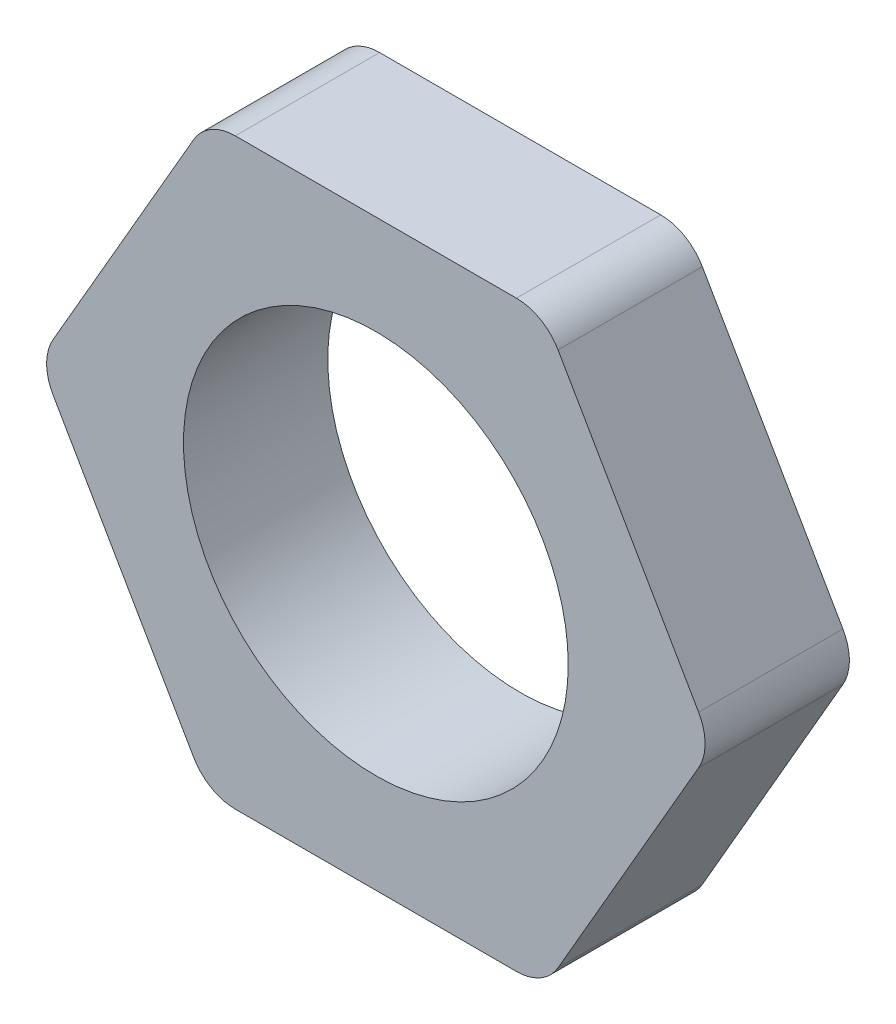
ISO-10303-21;
HEADER;
FILE_DESCRIPTION(('STEP AP214'),'2;1');
FILE_NAME('part.step','',(''),(''),'','','');
FILE_SCHEMA(('AUTOMOTIVE_DESIGN { 1 0 10303 214 1 1 1 1 }'));
ENDSEC;
DATA;
#1=APPLICATION_CONTEXT('core data for automotive mechanical design processes');
#2=APPLICATION_PROTOCOL_DEFINITION('international standard','automotive_design',2000,#1);
#3=PRODUCT_CONTEXT('',#1,'mechanical');
#4=PRODUCT('Part','Part','',(#3));
#5=PRODUCT_RELATED_PRODUCT_CATEGORY('part','',(#4));
#6=PRODUCT_DEFINITION_FORMATION('','',#4);
#7=PRODUCT_DEFINITION_CONTEXT('part definition',#1,'design');
#8=PRODUCT_DEFINITION('design','',#6,#7);
#9=PRODUCT_DEFINITION_SHAPE('','',#8);
#10=(LENGTH_UNIT() NAMED_UNIT(*) SI_UNIT(.MILLI.,.METRE.));
#11=(NAMED_UNIT(*) PLANE_ANGLE_UNIT() SI_UNIT($,.RADIAN.));
#12=(NAMED_UNIT(*) SI_UNIT($,.STERADIAN.) SOLID_ANGLE_UNIT());
#13=UNCERTAINTY_MEASURE_WITH_UNIT(LENGTH_MEASURE(1.E-05),#10,'distance_accuracy_value','');
#14=(GEOMETRIC_REPRESENTATION_CONTEXT(3) GLOBAL_UNCERTAINTY_ASSIGNED_CONTEXT((#13)) GLOBAL_UNIT_ASSIGNED_CONTEXT((#10,
#11,#12)) REPRESENTATION_CONTEXT('',''));
#15=CARTESIAN_POINT('',(0.,0.,0.));
#16=DIRECTION('',(0.,0.,1.));
#17=DIRECTION('',(1.,0.,0.));
#18=AXIS2_PLACEMENT_3D('',#15,#16,#17);
#19=CARTESIAN_POINT('',(-3.5,-6.06217782649107,3.));
#20=DIRECTION('',(0.,1.,0.));
#21=DIRECTION('',(-1.,0.,0.));
#22=AXIS2_PLACEMENT_3D('',#19,#20,#21);
#23=PLANE('',#22);
#24=DIRECTION('',(1.,0.,0.));
#25=VECTOR('',#24,1.);
#26=CARTESIAN_POINT('',(-3.5,-6.06217782649107,0.));
#27=LINE('',#26,#25);
#28=CARTESIAN_POINT('',(-2.92264973081037,-6.06217782649107,0.));
#29=VERTEX_POINT('',#28);
#30=CARTESIAN_POINT('',(2.92264973081038,-6.06217782649107,0.));
#31=VERTEX_POINT('',#30);
#32=EDGE_CURVE('E164',#29,#31,#27,.T.);
#33=ORIENTED_EDGE('',*,*,#32,.T.);
#34=DIRECTION('',(0.,0.,-1.));
#35=VECTOR('',#34,1.);
#36=CARTESIAN_POINT('',(2.92264973081038,-6.06217782649107,3.));
#37=LINE('',#36,#35);
#38=CARTESIAN_POINT('',(2.92264973081038,-6.06217782649107,3.));
#39=VERTEX_POINT('',#38);
#40=EDGE_CURVE('E203',#31,#39,#37,.F.);
#41=ORIENTED_EDGE('',*,*,#40,.T.);
#42=DIRECTION('',(1.,0.,0.));
#43=VECTOR('',#42,1.);
#44=CARTESIAN_POINT('',(-3.5,-6.06217782649107,3.));
#45=LINE('',#44,#43);
#46=CARTESIAN_POINT('',(-2.92264973081037,-6.06217782649107,3.));
#47=VERTEX_POINT('',#46);
#48=EDGE_CURVE('E174',#47,#39,#45,.T.);
#49=ORIENTED_EDGE('',*,*,#48,.F.);
#50=DIRECTION('',(0.,0.,-1.));
#51=VECTOR('',#50,1.);
#52=CARTESIAN_POINT('',(-2.92264973081037,-6.06217782649107,3.));
#53=LINE('',#52,#51);
#54=EDGE_CURVE('E196',#47,#29,#53,.T.);
#55=ORIENTED_EDGE('',*,*,#54,.T.);
#56=EDGE_LOOP('',(#33,#41,#49,#55));
#57=FACE_BOUND('',#56,.T.);
#58=ADVANCED_FACE('F43',(#57),#23,.F.);
#59=CARTESIAN_POINT('',(3.5,-6.06217782649107,3.));
#60=DIRECTION('',(-0.866025403784439,0.5,0.));
#61=DIRECTION('',(-0.5,-0.866025403784439,0.));
#62=AXIS2_PLACEMENT_3D('',#59,#60,#61);
#63=PLANE('',#62);
#64=DIRECTION('',(0.5,0.866025403784439,0.));
#65=VECTOR('',#64,1.);
#66=CARTESIAN_POINT('',(3.5,-6.06217782649107,0.));
#67=LINE('',#66,#65);
#68=CARTESIAN_POINT('',(3.78867513459481,-5.56217782649107,0.));
#69=VERTEX_POINT('',#68);
#70=CARTESIAN_POINT('',(6.71132486540519,-0.5,0.));
#71=VERTEX_POINT('',#70);
#72=EDGE_CURVE('E159',#69,#71,#67,.T.);
#73=ORIENTED_EDGE('',*,*,#72,.T.);
#74=DIRECTION('',(0.,0.,-1.));
#75=VECTOR('',#74,1.);
#76=CARTESIAN_POINT('',(6.71132486540519,-0.5,3.));
#77=LINE('',#76,#75);
#78=CARTESIAN_POINT('',(6.71132486540519,-0.5,3.));
#79=VERTEX_POINT('',#78);
#80=EDGE_CURVE('E136',#71,#79,#77,.F.);
#81=ORIENTED_EDGE('',*,*,#80,.T.);
#82=DIRECTION('',(0.5,0.866025403784439,0.));
#83=VECTOR('',#82,1.);
#84=CARTESIAN_POINT('',(3.5,-6.06217782649107,3.));
#85=LINE('',#84,#83);
#86=CARTESIAN_POINT('',(3.78867513459481,-5.56217782649107,3.));
#87=VERTEX_POINT('',#86);
#88=EDGE_CURVE('E249',#87,#79,#85,.T.);
#89=ORIENTED_EDGE('',*,*,#88,.F.);
#90=DIRECTION('',(0.,0.,-1.));
#91=VECTOR('',#90,1.);
#92=CARTESIAN_POINT('',(3.78867513459481,-5.56217782649107,3.));
#93=LINE('',#92,#91);
#94=EDGE_CURVE('E141',#87,#69,#93,.T.);
#95=ORIENTED_EDGE('',*,*,#94,.T.);
#96=EDGE_LOOP('',(#73,#81,#89,#95));
#97=FACE_BOUND('',#96,.T.);
#98=ADVANCED_FACE('F262',(#97),#63,.F.);
#99=CARTESIAN_POINT('',(7.,0.,3.));
#100=DIRECTION('',(-0.866025403784439,-0.5,0.));
#101=DIRECTION('',(0.5,-0.866025403784439,0.));
#102=AXIS2_PLACEMENT_3D('',#99,#100,#101);
#103=PLANE('',#102);
#104=DIRECTION('',(-0.5,0.866025403784438,0.));
#105=VECTOR('',#104,1.);
#106=CARTESIAN_POINT('',(7.,0.,3.));
#107=LINE('',#106,#105);
#108=CARTESIAN_POINT('',(6.71132486540519,0.5,3.));
#109=VERTEX_POINT('',#108);
#110=CARTESIAN_POINT('',(3.78867513459481,5.56217782649107,3.));
#111=VERTEX_POINT('',#110);
#112=EDGE_CURVE('E153',#109,#111,#107,.T.);
#113=ORIENTED_EDGE('',*,*,#112,.F.);
#114=DIRECTION('',(0.,0.,-1.));
#115=VECTOR('',#114,1.);
#116=CARTESIAN_POINT('',(6.71132486540519,0.5,3.));
#117=LINE('',#116,#115);
#118=CARTESIAN_POINT('',(6.71132486540519,0.5,0.));
#119=VERTEX_POINT('',#118);
#120=EDGE_CURVE('E140',#109,#119,#117,.T.);
#121=ORIENTED_EDGE('',*,*,#120,.T.);
#122=DIRECTION('',(-0.5,0.866025403784438,0.));
#123=VECTOR('',#122,1.);
#124=CARTESIAN_POINT('',(7.,0.,0.));
#125=LINE('',#124,#123);
#126=CARTESIAN_POINT('',(3.78867513459481,5.56217782649107,0.));
#127=VERTEX_POINT('',#126);
#128=EDGE_CURVE('E147',#119,#127,#125,.T.);
#129=ORIENTED_EDGE('',*,*,#128,.T.);
#130=DIRECTION('',(0.,0.,-1.));
#131=VECTOR('',#130,1.);
#132=CARTESIAN_POINT('',(3.78867513459481,5.56217782649107,3.));
#133=LINE('',#132,#131);
#134=EDGE_CURVE('E154',#127,#111,#133,.F.);
#135=ORIENTED_EDGE('',*,*,#134,.T.);
#136=EDGE_LOOP('',(#113,#121,#129,#135));
#137=FACE_BOUND('',#136,.T.);
#138=ADVANCED_FACE('F149',(#137),#103,.F.);
#139=CARTESIAN_POINT('',(3.5,6.06217782649107,3.));
#140=DIRECTION('',(0.,-1.,0.));
#141=DIRECTION('',(0.,0.,-1.));
#142=AXIS2_PLACEMENT_3D('',#139,#140,#141);
#143=PLANE('',#142);
#144=DIRECTION('',(-1.,0.,0.));
#145=VECTOR('',#144,1.);
#146=CARTESIAN_POINT('',(3.5,6.06217782649107,0.));
#147=LINE('',#146,#145);
#148=CARTESIAN_POINT('',(2.92264973081037,6.06217782649107,0.));
#149=VERTEX_POINT('',#148);
#150=CARTESIAN_POINT('',(-2.92264973081037,6.06217782649107,0.));
#151=VERTEX_POINT('',#150);
#152=EDGE_CURVE('E157',#149,#151,#147,.T.);
#153=ORIENTED_EDGE('',*,*,#152,.T.);
#154=DIRECTION('',(0.,0.,-1.));
#155=VECTOR('',#154,1.);
#156=CARTESIAN_POINT('',(-2.92264973081037,6.06217782649107,3.));
#157=LINE('',#156,#155);
#158=CARTESIAN_POINT('',(-2.92264973081037,6.06217782649107,3.));
#159=VERTEX_POINT('',#158);
#160=EDGE_CURVE('E11',#151,#159,#157,.F.);
#161=ORIENTED_EDGE('',*,*,#160,.T.);
#162=DIRECTION('',(-1.,0.,0.));
#163=VECTOR('',#162,1.);
#164=CARTESIAN_POINT('',(3.5,6.06217782649107,3.));
#165=LINE('',#164,#163);
#166=CARTESIAN_POINT('',(2.92264973081037,6.06217782649107,3.));
#167=VERTEX_POINT('',#166);
#168=EDGE_CURVE('E217',#167,#159,#165,.T.);
#169=ORIENTED_EDGE('',*,*,#168,.F.);
#170=DIRECTION('',(0.,0.,-1.));
#171=VECTOR('',#170,1.);
#172=CARTESIAN_POINT('',(2.92264973081037,6.06217782649107,3.));
#173=LINE('',#172,#171);
#174=EDGE_CURVE('E51',#167,#149,#173,.T.);
#175=ORIENTED_EDGE('',*,*,#174,.T.);
#176=EDGE_LOOP('',(#153,#161,#169,#175));
#177=FACE_BOUND('',#176,.T.);
#178=ADVANCED_FACE('F214',(#177),#143,.F.);
#179=CARTESIAN_POINT('',(-3.5,6.06217782649107,3.));
#180=DIRECTION('',(0.866025403784439,-0.5,0.));
#181=DIRECTION('',(0.5,0.866025403784439,0.));
#182=AXIS2_PLACEMENT_3D('',#179,#180,#181);
#183=PLANE('',#182);
#184=DIRECTION('',(-0.5,-0.866025403784439,0.));
#185=VECTOR('',#184,1.);
#186=CARTESIAN_POINT('',(-3.5,6.06217782649107,0.));
#187=LINE('',#186,#185);
#188=CARTESIAN_POINT('',(-3.78867513459481,5.56217782649107,0.));
#189=VERTEX_POINT('',#188);
#190=CARTESIAN_POINT('',(-6.71132486540519,0.5,0.));
#191=VERTEX_POINT('',#190);
#192=EDGE_CURVE('E162',#189,#191,#187,.T.);
#193=ORIENTED_EDGE('',*,*,#192,.T.);
#194=DIRECTION('',(0.,0.,-1.));
#195=VECTOR('',#194,1.);
#196=CARTESIAN_POINT('',(-6.71132486540519,0.5,3.));
#197=LINE('',#196,#195);
#198=CARTESIAN_POINT('',(-6.71132486540519,0.5,3.));
#199=VERTEX_POINT('',#198);
#200=EDGE_CURVE('E209',#191,#199,#197,.F.);
#201=ORIENTED_EDGE('',*,*,#200,.T.);
#202=DIRECTION('',(-0.5,-0.866025403784439,0.));
#203=VECTOR('',#202,1.);
#204=CARTESIAN_POINT('',(-3.5,6.06217782649107,3.));
#205=LINE('',#204,#203);
#206=CARTESIAN_POINT('',(-3.78867513459481,5.56217782649107,3.));
#207=VERTEX_POINT('',#206);
#208=EDGE_CURVE('E230',#207,#199,#205,.T.);
#209=ORIENTED_EDGE('',*,*,#208,.F.);
#210=DIRECTION('',(0.,0.,-1.));
#211=VECTOR('',#210,1.);
#212=CARTESIAN_POINT('',(-3.78867513459481,5.56217782649107,3.));
#213=LINE('',#212,#211);
#214=EDGE_CURVE('E210',#207,#189,#213,.T.);
#215=ORIENTED_EDGE('',*,*,#214,.T.);
#216=EDGE_LOOP('',(#193,#201,#209,#215));
#217=FACE_BOUND('',#216,.T.);
#218=ADVANCED_FACE('F229',(#217),#183,.F.);
#219=CARTESIAN_POINT('',(-7.,0.,3.));
#220=DIRECTION('',(0.866025403784439,0.5,0.));
#221=DIRECTION('',(-0.5,0.866025403784439,0.));
#222=AXIS2_PLACEMENT_3D('',#219,#220,#221);
#223=PLANE('',#222);
#224=DIRECTION('',(0.5,-0.866025403784439,0.));
#225=VECTOR('',#224,1.);
#226=CARTESIAN_POINT('',(-7.,0.,0.));
#227=LINE('',#226,#225);
#228=CARTESIAN_POINT('',(-6.71132486540519,-0.499999999999999,0.));
#229=VERTEX_POINT('',#228);
#230=CARTESIAN_POINT('',(-3.78867513459481,-5.56217782649107,0.));
#231=VERTEX_POINT('',#230);
#232=EDGE_CURVE('E171',#229,#231,#227,.T.);
#233=ORIENTED_EDGE('',*,*,#232,.T.);
#234=DIRECTION('',(0.,0.,-1.));
#235=VECTOR('',#234,1.);
#236=CARTESIAN_POINT('',(-3.78867513459481,-5.56217782649107,3.));
#237=LINE('',#236,#235);
#238=CARTESIAN_POINT('',(-3.78867513459481,-5.56217782649107,3.));
#239=VERTEX_POINT('',#238);
#240=EDGE_CURVE('E59',#231,#239,#237,.F.);
#241=ORIENTED_EDGE('',*,*,#240,.T.);
#242=DIRECTION('',(0.5,-0.866025403784439,0.));
#243=VECTOR('',#242,1.);
#244=CARTESIAN_POINT('',(-7.,0.,3.));
#245=LINE('',#244,#243);
#246=CARTESIAN_POINT('',(-6.71132486540519,-0.499999999999999,3.));
#247=VERTEX_POINT('',#246);
#248=EDGE_CURVE('E173',#247,#239,#245,.T.);
#249=ORIENTED_EDGE('',*,*,#248,.F.);
#250=DIRECTION('',(0.,0.,-1.));
#251=VECTOR('',#250,1.);
#252=CARTESIAN_POINT('',(-6.71132486540519,-0.499999999999999,3.));
#253=LINE('',#252,#251);
#254=EDGE_CURVE('E201',#247,#229,#253,.T.);
#255=ORIENTED_EDGE('',*,*,#254,.T.);
#256=EDGE_LOOP('',(#233,#241,#249,#255));
#257=FACE_BOUND('',#256,.T.);
#258=ADVANCED_FACE('F287',(#257),#223,.F.);
#259=CARTESIAN_POINT('',(0.,0.,3.));
#260=DIRECTION('',(0.,0.,1.));
#261=DIRECTION('',(1.,0.,0.));
#262=AXIS2_PLACEMENT_3D('',#259,#260,#261);
#263=PLANE('',#262);
#264=CARTESIAN_POINT('',(0.,0.,3.));
#265=DIRECTION('',(0.,0.,1.));
#266=DIRECTION('',(1.,0.,0.));
#267=AXIS2_PLACEMENT_3D('',#264,#265,#266);
#268=CIRCLE('',#267,4.);
#269=CARTESIAN_POINT('',(4.,0.,3.));
#270=VERTEX_POINT('',#269);
#271=EDGE_CURVE('E241',#270,#270,#268,.T.);
#272=ORIENTED_EDGE('',*,*,#271,.F.);
#273=EDGE_LOOP('',(#272));
#274=FACE_BOUND('',#273,.T.);
#275=ORIENTED_EDGE('',*,*,#88,.T.);
#276=CARTESIAN_POINT('',(5.84529946162075,0.,3.));
#277=DIRECTION('',(0.,0.,1.));
#278=DIRECTION('',(1.,0.,0.));
#279=AXIS2_PLACEMENT_3D('',#276,#277,#278);
#280=CIRCLE('',#279,1.);
#281=EDGE_CURVE('E198',#79,#109,#280,.T.);
#282=ORIENTED_EDGE('',*,*,#281,.T.);
#283=ORIENTED_EDGE('',*,*,#112,.T.);
#284=CARTESIAN_POINT('',(2.92264973081037,5.06217782649107,3.));
#285=DIRECTION('',(0.,0.,1.));
#286=DIRECTION('',(1.,0.,0.));
#287=AXIS2_PLACEMENT_3D('',#284,#285,#286);
#288=CIRCLE('',#287,1.);
#289=EDGE_CURVE('E187',#111,#167,#288,.T.);
#290=ORIENTED_EDGE('',*,*,#289,.T.);
#291=ORIENTED_EDGE('',*,*,#168,.T.);
#292=CARTESIAN_POINT('',(-2.92264973081037,5.06217782649107,3.));
#293=DIRECTION('',(0.,0.,1.));
#294=DIRECTION('',(1.,0.,0.));
#295=AXIS2_PLACEMENT_3D('',#292,#293,#294);
#296=CIRCLE('',#295,1.);
#297=EDGE_CURVE('E188',#159,#207,#296,.T.);
#298=ORIENTED_EDGE('',*,*,#297,.T.);
#299=ORIENTED_EDGE('',*,*,#208,.T.);
#300=CARTESIAN_POINT('',(-5.84529946162075,0.,3.));
#301=DIRECTION('',(0.,0.,1.));
#302=DIRECTION('',(1.,0.,0.));
#303=AXIS2_PLACEMENT_3D('',#300,#301,#302);
#304=CIRCLE('',#303,1.);
#305=EDGE_CURVE('E65',#199,#247,#304,.T.);
#306=ORIENTED_EDGE('',*,*,#305,.T.);
#307=ORIENTED_EDGE('',*,*,#248,.T.);
#308=CARTESIAN_POINT('',(-2.92264973081037,-5.06217782649107,3.));
#309=DIRECTION('',(0.,0.,1.));
#310=DIRECTION('',(1.,0.,0.));
#311=AXIS2_PLACEMENT_3D('',#308,#309,#310);
#312=CIRCLE('',#311,1.);
#313=EDGE_CURVE('E195',#239,#47,#312,.T.);
#314=ORIENTED_EDGE('',*,*,#313,.T.);
#315=ORIENTED_EDGE('',*,*,#48,.T.);
#316=CARTESIAN_POINT('',(2.92264973081038,-5.06217782649107,3.));
#317=DIRECTION('',(0.,0.,1.));
#318=DIRECTION('',(1.,0.,0.));
#319=AXIS2_PLACEMENT_3D('',#316,#317,#318);
#320=CIRCLE('',#319,1.);
#321=EDGE_CURVE('E192',#39,#87,#320,.T.);
#322=ORIENTED_EDGE('',*,*,#321,.T.);
#323=EDGE_LOOP('',(#275,#282,#283,#290,#291,#298,#299,#306,#307,#314,#315,#322));
#324=FACE_BOUND('',#323,.T.);
#325=ADVANCED_FACE('F252',(#274,#324),#263,.T.);
#326=CARTESIAN_POINT('',(0.,0.,0.));
#327=DIRECTION('',(0.,0.,1.));
#328=DIRECTION('',(1.,0.,0.));
#329=AXIS2_PLACEMENT_3D('',#326,#327,#328);
#330=PLANE('',#329);
#331=CARTESIAN_POINT('',(0.,0.,0.));
#332=DIRECTION('',(0.,0.,1.));
#333=DIRECTION('',(1.,0.,0.));
#334=AXIS2_PLACEMENT_3D('',#331,#332,#333);
#335=CIRCLE('',#334,4.);
#336=CARTESIAN_POINT('',(4.,0.,0.));
#337=VERTEX_POINT('',#336);
#338=EDGE_CURVE('E237',#337,#337,#335,.T.);
#339=ORIENTED_EDGE('',*,*,#338,.T.);
#340=EDGE_LOOP('',(#339));
#341=FACE_BOUND('',#340,.T.);
#342=ORIENTED_EDGE('',*,*,#128,.F.);
#343=CARTESIAN_POINT('',(5.84529946162075,0.,0.));
#344=DIRECTION('',(0.,0.,1.));
#345=DIRECTION('',(1.,0.,0.));
#346=AXIS2_PLACEMENT_3D('',#343,#344,#345);
#347=CIRCLE('',#346,1.);
#348=EDGE_CURVE('E134',#119,#71,#347,.F.);
#349=ORIENTED_EDGE('',*,*,#348,.T.);
#350=ORIENTED_EDGE('',*,*,#72,.F.);
#351=CARTESIAN_POINT('',(2.92264973081038,-5.06217782649107,0.));
#352=DIRECTION('',(0.,0.,1.));
#353=DIRECTION('',(1.,0.,0.));
#354=AXIS2_PLACEMENT_3D('',#351,#352,#353);
#355=CIRCLE('',#354,1.);
#356=EDGE_CURVE('E145',#69,#31,#355,.F.);
#357=ORIENTED_EDGE('',*,*,#356,.T.);
#358=ORIENTED_EDGE('',*,*,#32,.F.);
#359=CARTESIAN_POINT('',(-2.92264973081037,-5.06217782649107,0.));
#360=DIRECTION('',(0.,0.,1.));
#361=DIRECTION('',(1.,0.,0.));
#362=AXIS2_PLACEMENT_3D('',#359,#360,#361);
#363=CIRCLE('',#362,1.);
#364=EDGE_CURVE('E182',#29,#231,#363,.F.);
#365=ORIENTED_EDGE('',*,*,#364,.T.);
#366=ORIENTED_EDGE('',*,*,#232,.F.);
#367=CARTESIAN_POINT('',(-5.84529946162075,0.,0.));
#368=DIRECTION('',(0.,0.,1.));
#369=DIRECTION('',(1.,0.,0.));
#370=AXIS2_PLACEMENT_3D('',#367,#368,#369);
#371=CIRCLE('',#370,1.);
#372=EDGE_CURVE('E177',#229,#191,#371,.F.);
#373=ORIENTED_EDGE('',*,*,#372,.T.);
#374=ORIENTED_EDGE('',*,*,#192,.F.);
#375=CARTESIAN_POINT('',(-2.92264973081037,5.06217782649107,0.));
#376=DIRECTION('',(0.,0.,1.));
#377=DIRECTION('',(1.,0.,0.));
#378=AXIS2_PLACEMENT_3D('',#375,#376,#377);
#379=CIRCLE('',#378,1.);
#380=EDGE_CURVE('E180',#189,#151,#379,.F.);
#381=ORIENTED_EDGE('',*,*,#380,.T.);
#382=ORIENTED_EDGE('',*,*,#152,.F.);
#383=CARTESIAN_POINT('',(2.92264973081037,5.06217782649107,0.));
#384=DIRECTION('',(0.,0.,1.));
#385=DIRECTION('',(1.,0.,0.));
#386=AXIS2_PLACEMENT_3D('',#383,#384,#385);
#387=CIRCLE('',#386,1.);
#388=EDGE_CURVE('E152',#149,#127,#387,.F.);
#389=ORIENTED_EDGE('',*,*,#388,.T.);
#390=EDGE_LOOP('',(#342,#349,#350,#357,#358,#365,#366,#373,#374,#381,#382,#389));
#391=FACE_BOUND('',#390,.T.);
#392=ADVANCED_FACE('F160',(#341,#391),#330,.F.);
#393=CARTESIAN_POINT('',(5.84529946162075,0.,3.));
#394=DIRECTION('',(0.,0.,-1.));
#395=DIRECTION('',(-1.,0.,0.));
#396=AXIS2_PLACEMENT_3D('',#393,#394,#395);
#397=CYLINDRICAL_SURFACE('',#396,1.);
#398=ORIENTED_EDGE('',*,*,#281,.F.);
#399=ORIENTED_EDGE('',*,*,#80,.F.);
#400=ORIENTED_EDGE('',*,*,#348,.F.);
#401=ORIENTED_EDGE('',*,*,#120,.F.);
#402=EDGE_LOOP('',(#398,#399,#400,#401));
#403=FACE_BOUND('',#402,.T.);
#404=ADVANCED_FACE('F138',(#403),#397,.T.);
#405=CARTESIAN_POINT('',(2.92264973081038,-5.06217782649107,3.));
#406=DIRECTION('',(0.,0.,-1.));
#407=DIRECTION('',(-1.,0.,0.));
#408=AXIS2_PLACEMENT_3D('',#405,#406,#407);
#409=CYLINDRICAL_SURFACE('',#408,1.);
#410=ORIENTED_EDGE('',*,*,#321,.F.);
#411=ORIENTED_EDGE('',*,*,#40,.F.);
#412=ORIENTED_EDGE('',*,*,#356,.F.);
#413=ORIENTED_EDGE('',*,*,#94,.F.);
#414=EDGE_LOOP('',(#410,#411,#412,#413));
#415=FACE_BOUND('',#414,.T.);
#416=ADVANCED_FACE('F274',(#415),#409,.T.);
#417=CARTESIAN_POINT('',(-2.92264973081037,-5.06217782649107,3.));
#418=DIRECTION('',(0.,0.,-1.));
#419=DIRECTION('',(-1.,0.,0.));
#420=AXIS2_PLACEMENT_3D('',#417,#418,#419);
#421=CYLINDRICAL_SURFACE('',#420,1.);
#422=ORIENTED_EDGE('',*,*,#313,.F.);
#423=ORIENTED_EDGE('',*,*,#240,.F.);
#424=ORIENTED_EDGE('',*,*,#364,.F.);
#425=ORIENTED_EDGE('',*,*,#54,.F.);
#426=EDGE_LOOP('',(#422,#423,#424,#425));
#427=FACE_BOUND('',#426,.T.);
#428=ADVANCED_FACE('F279',(#427),#421,.T.);
#429=CARTESIAN_POINT('',(-5.84529946162075,0.,3.));
#430=DIRECTION('',(0.,0.,-1.));
#431=DIRECTION('',(-1.,0.,0.));
#432=AXIS2_PLACEMENT_3D('',#429,#430,#431);
#433=CYLINDRICAL_SURFACE('',#432,1.);
#434=ORIENTED_EDGE('',*,*,#305,.F.);
#435=ORIENTED_EDGE('',*,*,#200,.F.);
#436=ORIENTED_EDGE('',*,*,#372,.F.);
#437=ORIENTED_EDGE('',*,*,#254,.F.);
#438=EDGE_LOOP('',(#434,#435,#436,#437));
#439=FACE_BOUND('',#438,.T.);
#440=ADVANCED_FACE('F265',(#439),#433,.T.);
#441=CARTESIAN_POINT('',(-2.92264973081037,5.06217782649107,3.));
#442=DIRECTION('',(0.,0.,-1.));
#443=DIRECTION('',(-1.,0.,0.));
#444=AXIS2_PLACEMENT_3D('',#441,#442,#443);
#445=CYLINDRICAL_SURFACE('',#444,1.);
#446=ORIENTED_EDGE('',*,*,#297,.F.);
#447=ORIENTED_EDGE('',*,*,#160,.F.);
#448=ORIENTED_EDGE('',*,*,#380,.F.);
#449=ORIENTED_EDGE('',*,*,#214,.F.);
#450=EDGE_LOOP('',(#446,#447,#448,#449));
#451=FACE_BOUND('',#450,.T.);
#452=ADVANCED_FACE('F223',(#451),#445,.T.);
#453=CARTESIAN_POINT('',(2.92264973081037,5.06217782649107,3.));
#454=DIRECTION('',(0.,0.,-1.));
#455=DIRECTION('',(-1.,0.,0.));
#456=AXIS2_PLACEMENT_3D('',#453,#454,#455);
#457=CYLINDRICAL_SURFACE('',#456,1.);
#458=ORIENTED_EDGE('',*,*,#289,.F.);
#459=ORIENTED_EDGE('',*,*,#134,.F.);
#460=ORIENTED_EDGE('',*,*,#388,.F.);
#461=ORIENTED_EDGE('',*,*,#174,.F.);
#462=EDGE_LOOP('',(#458,#459,#460,#461));
#463=FACE_BOUND('',#462,.T.);
#464=ADVANCED_FACE('F44',(#463),#457,.T.);
#465=CARTESIAN_POINT('',(0.,0.,0.));
#466=DIRECTION('',(0.,0.,1.));
#467=DIRECTION('',(1.,0.,0.));
#468=AXIS2_PLACEMENT_3D('',#465,#466,#467);
#469=CYLINDRICAL_SURFACE('',#468,4.);
#470=ORIENTED_EDGE('',*,*,#338,.F.);
#471=EDGE_LOOP('',(#470));
#472=FACE_BOUND('',#471,.T.);
#473=ORIENTED_EDGE('',*,*,#271,.T.);
#474=EDGE_LOOP('',(#473));
#475=FACE_BOUND('',#474,.T.);
#476=ADVANCED_FACE('F255',(#472,#475),#469,.F.);
#477=CLOSED_SHELL('',(#58,#98,#138,#178,#218,#258,#325,#392,#404,#416,#428,#440,#452,#464,#476));
#478=MANIFOLD_SOLID_BREP('B2',#477);
#479=ADVANCED_BREP_SHAPE_REPRESENTATION('',(#18,#478),#14);
#480=SHAPE_DEFINITION_REPRESENTATION(#9,#479);
ENDSEC;
END-ISO-10303-21;
